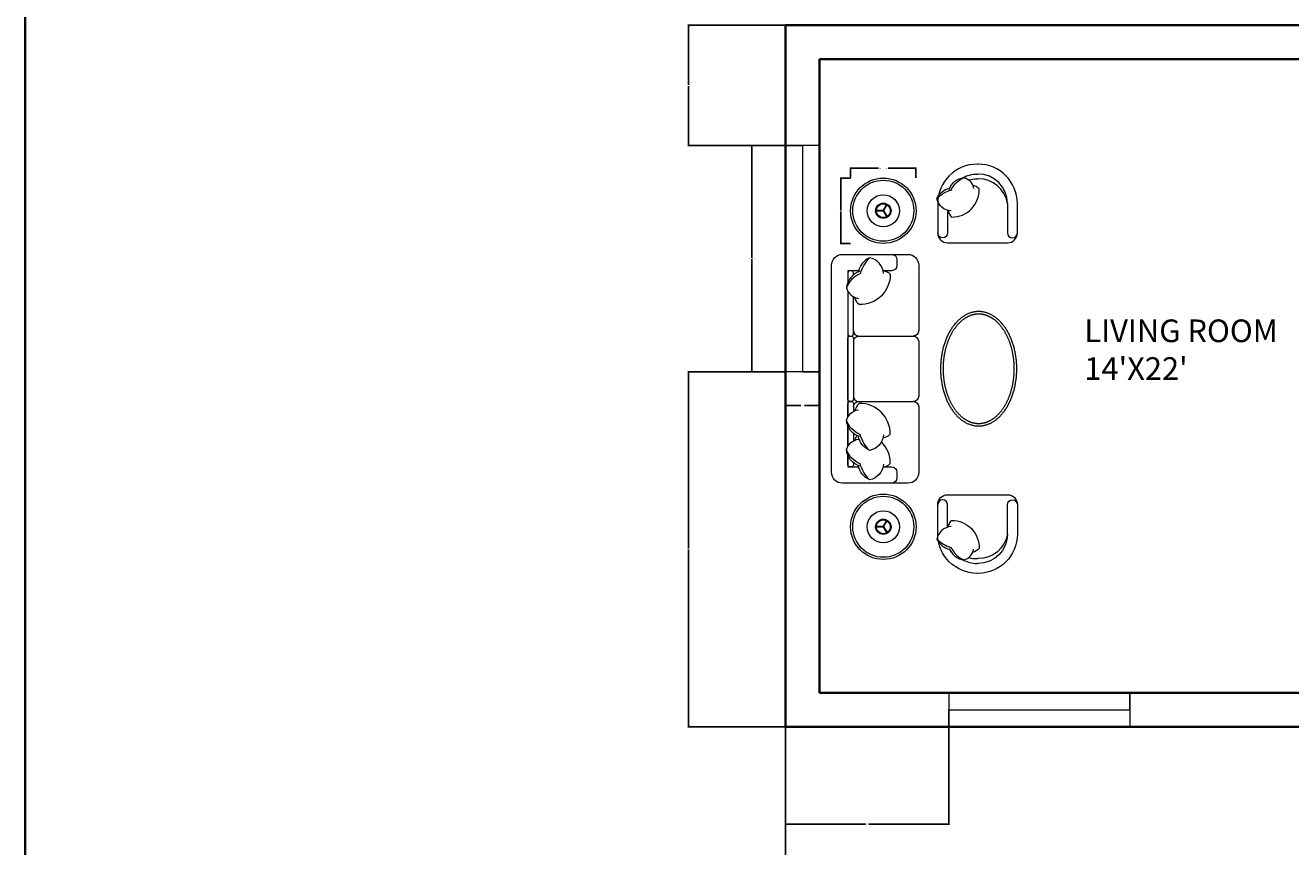
# Model space of a CAD drawing. Units: inches. Extents: x 2067 to 3463, y 1605 to 2723.
# Tile 2 of 10: x 2067 to 2403, y 1820 to 2038. Entities that reach past the tile are written whole.
import ezdxf

# ---------------------------------------------------------------- set-up
doc = ezdxf.new("R2010")
doc.units = ezdxf.units.IN
for name, color, linetype, lineweight in [('A-ANNO-DIMS', 2, 'Continuous', 18), ('A-ANNO-TTLB', 7, 'Continuous', 35), ('A-AREA-IDEN', 7, 'Continuous', 18), ('A-FURN', 8, 'Continuous', 13), ('A-GLAZ', 4, 'Continuous', 18), ('A-WALL', 7, 'Continuous', 35)]:
    doc.layers.add(name, color=color, linetype=linetype, lineweight=lineweight)
doc.styles.get("Standard").update_dxf_attribs({"font": 'arial.ttf'})
doc.dimstyles.get("Standard").update_dxf_attribs({"dimtxt": 0.18, "dimasz": 0.18, "dimexe": 0.18, "dimexo": 0.0625, "dimgap": 0.09, "dimtad": 0, "dimtih": 1, "dimtoh": 1, "dimdec": 4, "dimzin": 0, "dimdsep": 46, "dimtxsty": 'Standard', "dimcen": 0.09, "dimadec": 0, "dimazin": 0, "dimtfac": 1, "dimtdec": 4, "dimtofl": 0, "dimtmove": 0, "dimatfit": 3, "dimfxl": 1, "dimtolj": 1, "dimtzin": 0, "dimarcsym": 0})

# ---------------------------------------------------------------- blocks, each defined once
blk = doc.blocks.new('TABLE-SIDE-ROUND')
at = {"ltscale": 0.03}
for p, q in [((0, 0.09), (-2.04, 0.09)), ((-0.08, 0.05), (0.94, 1.81)), ((0.08, -0.05), (1.1, 1.72)), ((0.08, 0.05), (1.1, -1.72)), ((0, -0.09), (-2.04, -0.09)), ((-0.08, -0.05), (0.94, -1.81))]:
    blk.add_line(p, q, dxfattribs=at)
for radius in [8.67, 4.26, 2.04, 1.83]:
    blk.add_circle((0, 0), radius, dxfattribs=at)
blk.add_circle((0, 0), 8.09)
blk = doc.blocks.new('WIN-PLAN-60-OFFSET')
for p, q in [((0, 9), (0, 0)), ((60, 4.5), (60, 9)), ((60, 9), (60, 0)), ((0, 0), (0, 4.5)), ((0, 4.5), (60, 4.5))]:
    blk.add_line(p, q)
blk = doc.blocks.new('WIN-PLAN-48-OFFSET')
for p, q in [((0, 9), (0, 0)), ((48, 4.5), (48, 9)), ((48, 9), (48, 0)), ((0, 0), (0, 4.5)), ((0, 4.5), (48, 4.5))]:
    blk.add_line(p, q)
blk = doc.blocks.new('*D12')
at = {"layer": 'A-ANNO-DIMS', "color": 0, "lineweight": -2, "transparency": 16777216}
for p, q in [((2286.19, 1997.77), (2286.19, 2000.49)), ((2303.52, 1997.77), (2303.52, 2000.49)), ((2286.37, 2000.31), (2293.57, 2000.31)), ((2303.34, 2000.31), (2296.14, 2000.31))]:
    blk.add_line(p, q, dxfattribs=at)
at = {"layer": 'A-ANNO-DIMS', "color": 0, "transparency": 16777216}
for points in [[(2286.37, 2000.34), (2286.37, 2000.28), (2286.19, 2000.31)], [(2303.34, 2000.34), (2303.34, 2000.28), (2303.52, 2000.31)]]:
    blk.add_solid(points, dxfattribs=at)
at = {"layer": 'Defpoints', "color": 0, "transparency": 16777216}
for p in [(2286.19, 1997.71), (2303.52, 2000.31), (2303.52, 1997.71)]:
    blk.add_point(p, dxfattribs=at)
at = {"layer": 'A-ANNO-DIMS', "color": 0, "transparency": 16777216, "insert": (2294.86, 2000.31), "char_height": 0.18, "attachment_point": 5}
blk.add_mtext('\\A1;SIDE TABLE 17 TYP.', dxfattribs=at)
blk = doc.blocks.new('*D13')
at = {"layer": 'A-ANNO-DIMS', "color": 0, "lineweight": -2, "transparency": 16777216}
for p, q in [((2286.12, 1997.71), (2283.41, 1997.71)), ((2283.59, 1997.53), (2283.59, 1989.22)), ((2283.59, 1980.55), (2283.59, 1988.86)), ((2286.12, 1980.37), (2283.41, 1980.37))]:
    blk.add_line(p, q, dxfattribs=at)
at = {"layer": 'A-ANNO-DIMS', "color": 0, "transparency": 16777216}
for points in [[(2283.56, 1997.53), (2283.62, 1997.53), (2283.59, 1997.71)], [(2283.56, 1980.55), (2283.62, 1980.55), (2283.59, 1980.37)]]:
    blk.add_solid(points, dxfattribs=at)
at = {"layer": 'Defpoints', "color": 0, "transparency": 16777216}
for p in [(2283.59, 1997.71), (2286.19, 1997.71), (2286.19, 1980.37)]:
    blk.add_point(p, dxfattribs=at)
at = {"layer": 'A-ANNO-DIMS', "color": 0, "transparency": 16777216, "insert": (2283.59, 1989.04), "char_height": 0.18, "attachment_point": 5}
blk.add_mtext('\\A1;17 TYP.', dxfattribs=at)
blk = doc.blocks.new('*D22')
at = {"layer": 'A-ANNO-DIMS', "color": 0, "lineweight": -2, "transparency": 16777216}
for p, q in [((2268.89, 2006.36), (2259.77, 2006.36)), ((2259.95, 2006.18), (2259.95, 1976.54)), ((2259.95, 1946.54), (2259.95, 1976.18)), ((2268.89, 1946.36), (2259.77, 1946.36))]:
    blk.add_line(p, q, dxfattribs=at)
at = {"layer": 'A-ANNO-DIMS', "color": 0, "transparency": 16777216}
for points in [[(2259.92, 2006.18), (2259.98, 2006.18), (2259.95, 2006.36)], [(2259.92, 1946.54), (2259.98, 1946.54), (2259.95, 1946.36)]]:
    blk.add_solid(points, dxfattribs=at)
at = {"layer": 'Defpoints', "color": 0, "transparency": 16777216}
for p in [(2268.95, 2006.36), (2259.95, 1946.36), (2268.95, 1946.36)]:
    blk.add_point(p, dxfattribs=at)
at = {"layer": 'A-ANNO-DIMS', "color": 0, "transparency": 16777216, "insert": (2259.95, 1976.36), "char_height": 0.18, "attachment_point": 5}
blk.add_mtext('\\A1;WINDOW 60 TYP.', dxfattribs=at)
blk = doc.blocks.new('*D23')
at = {"layer": 'A-ANNO-DIMS', "color": 0, "lineweight": -2, "transparency": 16777216}
for p, q in [((2268.95, 1946.3), (2268.95, 1937.18)), ((2277.95, 1946.3), (2277.95, 1937.18)), ((2269.13, 1937.36), (2272.99, 1937.36)), ((2277.77, 1937.36), (2273.91, 1937.36))]:
    blk.add_line(p, q, dxfattribs=at)
at = {"layer": 'A-ANNO-DIMS', "color": 0, "transparency": 16777216}
for points in [[(2269.13, 1937.39), (2269.13, 1937.33), (2268.95, 1937.36)], [(2277.77, 1937.39), (2277.77, 1937.33), (2277.95, 1937.36)]]:
    blk.add_solid(points, dxfattribs=at)
at = {"layer": 'Defpoints', "color": 0, "transparency": 16777216}
for p in [(2268.95, 1946.36), (2277.95, 1946.36), (2277.95, 1937.36)]:
    blk.add_point(p, dxfattribs=at)
at = {"layer": 'A-ANNO-DIMS', "color": 0, "transparency": 16777216, "insert": (2273.45, 1937.36), "char_height": 0.18, "attachment_point": 5}
blk.add_mtext('\\A1;9 TYP.', dxfattribs=at)
blk = doc.blocks.new('*D32')
at = {"layer": 'A-ANNO-DIMS', "color": 0, "lineweight": -2, "transparency": 16777216}
for p, q in [((2268.89, 2038.22), (2242.97, 2038.22)), ((2243.15, 2038.04), (2243.15, 2022.47)), ((2243.15, 2006.54), (2243.15, 2022.11)), ((2268.89, 2006.36), (2242.97, 2006.36))]:
    blk.add_line(p, q, dxfattribs=at)
at = {"layer": 'A-ANNO-DIMS', "color": 0, "transparency": 16777216}
for points in [[(2243.12, 2038.04), (2243.18, 2038.04), (2243.15, 2038.22)], [(2243.12, 2006.54), (2243.18, 2006.54), (2243.15, 2006.36)]]:
    blk.add_solid(points, dxfattribs=at)
at = {"layer": 'Defpoints', "color": 0, "transparency": 16777216}
for p in [(2243.15, 2038.22), (2268.95, 2038.22), (2268.95, 2006.36)]:
    blk.add_point(p, dxfattribs=at)
at = {"layer": 'A-ANNO-DIMS', "color": 0, "transparency": 16777216, "insert": (2243.15, 2022.29), "char_height": 0.18, "attachment_point": 5}
blk.add_mtext('\\A1;31.86', dxfattribs=at)
blk = doc.blocks.new('*D33')
at = {"layer": 'A-ANNO-DIMS', "color": 0, "lineweight": -2, "transparency": 16777216}
for p, q in [((2268.89, 1946.36), (2242.97, 1946.36)), ((2243.15, 1946.18), (2243.15, 1899.47)), ((2243.15, 1852.4), (2243.15, 1899.11)), ((2268.89, 1852.22), (2242.97, 1852.22))]:
    blk.add_line(p, q, dxfattribs=at)
at = {"layer": 'A-ANNO-DIMS', "color": 0, "transparency": 16777216}
for points in [[(2243.12, 1946.18), (2243.18, 1946.18), (2243.15, 1946.36)], [(2243.12, 1852.4), (2243.18, 1852.4), (2243.15, 1852.22)]]:
    blk.add_solid(points, dxfattribs=at)
at = {"layer": 'Defpoints', "color": 0, "transparency": 16777216}
for p in [(2243.15, 1946.36), (2268.95, 1946.36), (2268.95, 1852.22)]:
    blk.add_point(p, dxfattribs=at)
at = {"layer": 'A-ANNO-DIMS', "color": 0, "transparency": 16777216, "insert": (2243.15, 1899.29), "char_height": 0.18, "attachment_point": 5}
blk.add_mtext('\\A1;94.14', dxfattribs=at)
blk = doc.blocks.new('*D36')
at = {"layer": 'A-ANNO-DIMS', "color": 0, "lineweight": -2, "transparency": 16777216}
for p, q in [((2268.95, 1852.15), (2268.95, 1764.75)), ((2433.25, 1806.19), (2433.25, 1764.75)), ((2269.13, 1764.93), (2350.71, 1764.93)), ((2433.07, 1764.93), (2351.49, 1764.93))]:
    blk.add_line(p, q, dxfattribs=at)
at = {"layer": 'A-ANNO-DIMS', "color": 0, "transparency": 16777216}
for points in [[(2269.13, 1764.96), (2269.13, 1764.9), (2268.95, 1764.93)], [(2433.07, 1764.96), (2433.07, 1764.9), (2433.25, 1764.93)]]:
    blk.add_solid(points, dxfattribs=at)
at = {"layer": 'Defpoints', "color": 0, "transparency": 16777216}
for p in [(2268.95, 1852.22), (2433.25, 1806.25), (2433.25, 1764.93)]:
    blk.add_point(p, dxfattribs=at)
at = {"layer": 'A-ANNO-DIMS', "color": 0, "transparency": 16777216, "insert": (2351.1, 1764.93), "char_height": 0.18, "attachment_point": 5}
blk.add_mtext('\\A1;164.3', dxfattribs=at)
blk = doc.blocks.new('*D42')
at = {"layer": 'A-ANNO-DIMS', "color": 0, "lineweight": -2, "transparency": 16777216}
for p, q in [((2268.95, 1852.15), (2268.95, 1826.24)), ((2312.26, 1852.15), (2312.26, 1826.24)), ((2269.13, 1826.42), (2290.22, 1826.42)), ((2312.08, 1826.42), (2290.98, 1826.42))]:
    blk.add_line(p, q, dxfattribs=at)
at = {"layer": 'A-ANNO-DIMS', "color": 0, "transparency": 16777216}
for points in [[(2269.13, 1826.45), (2269.13, 1826.39), (2268.95, 1826.42)], [(2312.08, 1826.45), (2312.08, 1826.39), (2312.26, 1826.42)]]:
    blk.add_solid(points, dxfattribs=at)
at = {"layer": 'Defpoints', "color": 0, "transparency": 16777216}
for p in [(2268.95, 1852.22), (2312.26, 1852.22), (2268.95, 1826.42)]:
    blk.add_point(p, dxfattribs=at)
at = {"layer": 'A-ANNO-DIMS', "color": 0, "transparency": 16777216, "insert": (2290.6, 1826.42), "char_height": 0.18, "attachment_point": 5}
blk.add_mtext('\\A1;43.31', dxfattribs=at)

msp = doc.modelspace()

# ---------------------------------------------------------------- linework, layer by layer
at = {"layer": 'A-ANNO-TTLB'}
msp.add_lwpolyline([(2067.2624, 2722.6321), (3463.3053, 2722.6321), (3463.3053, 1605.3918), (2067.2624, 1605.3918)], close=True, dxfattribs=at)
at = {"layer": 'A-FURN', "ltscale": 0.03}
for points in [[(2319.8521, 1980.5461), (2327.799, 1980.5461, 0.41421356), (2330.4045, 1983.1516), (2330.4045, 1990.9682, 0.41421356), (2319.9824, 2001.3903), (2319.8521, 2001.3903), (2319.7219, 2001.3903, 0.41421356), (2309.2997, 1990.9682), (2309.2997, 1983.1516, 0.41421356), (2311.9053, 1980.5461), (2319.8521, 1980.5461)], [(2319.8521, 1913.731), (2327.799, 1913.731, -0.41421356), (2330.4045, 1911.1254), (2330.4045, 1903.3089, -0.41421356), (2319.9824, 1892.8867), (2319.8521, 1892.8867), (2319.7219, 1892.8867, -0.41421356), (2309.2997, 1903.3089), (2309.2997, 1911.1254, -0.41421356), (2311.9053, 1913.731), (2319.8521, 1913.731)]]:
    msp.add_lwpolyline(points, format="xyb", dxfattribs=at)
at = {"layer": 'A-FURN'}
for points in [[(2309.0867, 1992.2833, -0.14772988), (2312.8943, 1994.5222, -0.21334276), (2316.2539, 1997.806, -0.17866181)], [(2312.3682, 1994.7007, -0.30666349), (2316.2539, 1997.806, -0.30632997), (2318.7923, 1994.97, 0.87284716)], [(2315.8418, 1997.7538, -0.13059149), (2319.7219, 1998.7848), (2319.8521, 1998.7848)], [(2317.5007, 1997.2013, -0.07238424), (2319.7219, 1997.482), (2319.8521, 1997.482)], [(2327.799, 1990.9682, 0.41421356), (2319.9824, 1998.7848), (2319.8521, 1998.7848)], [(2327.799, 1990.9682, 0.37271891), (2319.9824, 1997.482), (2319.8521, 1997.482)], [(2312.8196, 1988.9995, -0.35677236), (2309.0867, 1992.2833, -0.24954205), (2312.469, 1994.9894, 9.61688035)], [(2312.163, 1989.079, 0.16554063), (2312.9689, 1987.3576, 0.42598917), (2320.2855, 1994.8207, 0.12152332), (2318.5487, 1995.8494, -7.11546429)], [(2327.799, 1990.9683), (2327.799, 1983.1516, 0.41421356), (2329.1018, 1981.8489), (2329.1018, 1981.8489, 0.41421356), (2330.4045, 1983.1516)], [(2311.9053, 1989.1416), (2311.9053, 1983.1516, -0.41421356), (2310.6025, 1981.8489), (2310.6025, 1981.8489, -0.41421356), (2309.2997, 1983.1516)], [(2297.023, 1977.4811, -0.41421356), (2298.4678, 1976.0362), (2298.4678, 1974.5913, -0.41421356), (2297.023, 1973.1464), (2294.7843, 1973.1464)], [(2291.2298, 1976.5615, 0.14772988), (2288.7466, 1972.3385, 0.21334276), (2285.1046, 1968.6124, 0.17866181)], [(2294.8718, 1972.4213, 0.35677236), (2291.2298, 1976.5615, 0.24954205), (2288.2284, 1972.8101, -9.61688035)], [(2288.5487, 1972.922, 0.30666349), (2285.1046, 1968.6124, 0.30632997), (2288.2499, 1965.7971, -0.87284716)], [(2286.9088, 1972.0438), (2286.9088, 1972.5685, 0.41421356), (2286.3308, 1973.1464), (2286.0418, 1973.1464, 0.41421356), (2285.4639, 1972.5685)], [(2285.4639, 1972.5685), (2285.4639, 1970.1068, 0.41421356)], [(2294.7837, 1973.1496, -0.16554063), (2296.6928, 1972.2557, -0.42598917), (2288.4155, 1964.141, -0.12152332), (2287.2746, 1966.0673, 7.11546429)], [(2285.4639, 1967.703), (2285.4639, 1956.3858, 0.41421356), (2286.0418, 1955.8078), (2286.3308, 1955.8078, 0.41421356), (2286.9088, 1956.3858), (2286.9088, 1966.2481, 0.41421356)], [(2286.9088, 1957.2527, 0.41421356), (2288.3537, 1955.8078), (2302.8025, 1955.8078, 0.41421356)], [(2286.9088, 1954.363, -0.41421356), (2288.3537, 1955.8078)], [(2285.4639, 1934.3575), (2285.4639, 1937.8913, -0.41421356), (2286.0418, 1938.4692), (2286.3308, 1938.4692, -0.41421356), (2286.9088, 1937.8913), (2286.9088, 1935.8125, -0.41421356)], [(2286.9088, 1939.9141, 0.41421356), (2288.3537, 1938.4692)], [(2286.9088, 1937.0243, -0.41421356), (2288.3537, 1938.4692), (2302.8025, 1938.4692, -0.41421356)], [(2294.7837, 1928.911, 0.16554063), (2296.6928, 1929.8049, 0.42598917), (2288.4155, 1937.9196, 0.12152332), (2287.2746, 1935.9933, -7.11546429)], [(2288.5487, 1929.1386, -0.30666349), (2285.1046, 1933.4482, -0.30632997), (2288.2499, 1936.2635, 0.87284716)], [(2291.2298, 1925.4991, -0.14772988), (2288.7466, 1929.7221, -0.21334276), (2285.1046, 1933.4482, -0.17866181)], [(2285.4639, 1926.574), (2285.4639, 1931.9538, -0.41421356)], [(2286.9088, 1930.0168), (2286.9088, 1928.0289, -0.41421356)], [(2288.5487, 1921.3551, -0.30666349), (2285.1046, 1925.6647, -0.30632997), (2288.2499, 1928.48, 0.87284716)], [(2287.8395, 1929.4212, 0.07186538), (2287.2746, 1928.2098, -7.11546429)], [(2294.8718, 1929.6392, -0.35677236), (2291.2298, 1925.4991, -0.24954205), (2288.2284, 1929.2505, 9.61688035)], [(2294.7837, 1921.1275, 0.16554063), (2296.6928, 1922.0213, 0.20023115), (2294.3677, 1927.757, 0.12152332)], [(2291.2298, 1917.7155, -0.14772988), (2288.7466, 1921.9385, -0.21334276), (2285.1046, 1925.6647, -0.17866181)], [(2285.4639, 1924.1702), (2285.4639, 1921.1306), (2288.3034, 1921.1306, -0.41421356)], [(2285.4639, 1921.7086), (2285.4639, 1924.1702, -0.41421356)], [(2286.9088, 1922.2332), (2286.9088, 1921.7086, -0.41421356), (2286.3308, 1921.1306), (2286.0418, 1921.1306, -0.41421356), (2285.4639, 1921.7086)], [(2294.8718, 1921.8557, -0.35677236), (2291.2298, 1917.7155, -0.24954205), (2288.2284, 1921.4669, 9.61688035)], [(2294.7843, 1921.1306), (2297.023, 1921.1306, -0.41421356), (2298.4678, 1919.6857), (2298.4678, 1918.2408, -0.41421356), (2297.023, 1916.796)], [(2311.9053, 1905.1355), (2311.9053, 1911.1254, 0.41421356), (2310.6025, 1912.4282), (2310.6025, 1912.4282, 0.41421356), (2309.2997, 1911.1254)], [(2327.799, 1903.3087), (2327.799, 1911.1254, -0.41421356), (2329.1018, 1912.4282), (2329.1018, 1912.4282, -0.41421356), (2330.4045, 1911.1254)], [(2312.163, 1905.1981, -0.16554063), (2312.9689, 1906.9194, -0.42598917), (2320.2855, 1899.4563, -0.12152332), (2318.5487, 1898.4277, 7.11546429)], [(2312.8196, 1905.2775, 0.35677236), (2309.0867, 1901.9938, 0.24954205), (2312.469, 1899.2877, -9.61688035)], [(2327.799, 1903.3089, -0.37271891), (2319.9824, 1896.795), (2319.8521, 1896.795)], [(2327.799, 1903.3089, -0.41421356), (2319.9824, 1895.4923), (2319.8521, 1895.4923)], [(2309.0867, 1901.9938, 0.14772988), (2312.8943, 1899.7548, 0.21334276), (2316.2539, 1896.4711, 0.17866181)], [(2312.3682, 1899.5764, 0.30666349), (2316.2539, 1896.4711, 0.30632997), (2318.7923, 1899.307, -0.87284716)], [(2315.8418, 1896.5232, 0.13059149), (2319.7219, 1895.4923), (2319.8521, 1895.4923)], [(2317.5007, 1897.0757, 0.07238424), (2319.7219, 1896.795), (2319.8521, 1896.795)]]:
    msp.add_lwpolyline(points, format="xyb", dxfattribs=at)
at = {"layer": 'A-FURN', "ltscale": 0.03}
msp.add_lwpolyline([(2301.3576, 1977.4811, -0.41421356), (2304.2474, 1974.5913), (2304.2474, 1957.2527, -0.41421356), (2302.8025, 1955.8078, -0.41421356), (2304.2474, 1954.363), (2304.2474, 1939.9141, -0.41421356), (2302.8025, 1938.4692, -0.41421356), (2304.2474, 1937.0243), (2304.2474, 1919.6857, -0.41421356), (2301.3576, 1916.796), (2284.019, 1916.796, -0.41421356), (2281.1292, 1919.6857), (2281.1292, 1974.5913, -0.41421356), (2284.019, 1977.4811)], format="xyb", close=True, dxfattribs=at)
at = {"layer": 'A-FURN'}
for points in [[(2288.3034, 1973.1464), (2285.4639, 1973.1464), (2285.4639, 1970.1068)], [(2285.4639, 1967.703), (2285.4639, 1934.3575)], [(2285.4639, 1931.9538), (2285.4639, 1926.574)]]:
    msp.add_lwpolyline(points, dxfattribs=at)
msp.add_lwpolyline([(2285.4639, 1939.0472), (2285.4639, 1955.2299, -0.41421356), (2286.0418, 1955.8078), (2286.3308, 1955.8078, -0.41421356), (2286.9088, 1955.2299), (2286.9088, 1939.0472, -0.41421356), (2286.3308, 1938.4692), (2286.0418, 1938.4692, -0.41421356)], format="xyb", close=True, dxfattribs=at)
at = {"layer": 'A-FURN', "ltscale": 0.03}
msp.add_polyline3d([(2320.1411, 1962.3098, 0), (2319.9497, 1962.3071, 0), (2319.7584, 1962.2989, 0), (2319.5672, 1962.2854, 0), (2319.3762, 1962.2664, 0), (2319.1855, 1962.2419, 0), (2318.9951, 1962.2121, 0), (2318.8051, 1962.1769, 0), (2318.6156, 1962.1363, 0), (2318.4267, 1962.0903, 0), (2318.2384, 1962.0389, 0), (2318.0507, 1961.9823, 0), (2317.8638, 1961.9203, 0), (2317.6778, 1961.853, 0), (2317.4926, 1961.7804, 0), (2317.3083, 1961.7026, 0), (2317.1251, 1961.6196, 0), (2316.9429, 1961.5314, 0), (2316.7619, 1961.438, 0), (2316.5821, 1961.3395, 0), (2316.4036, 1961.236, 0), (2316.2264, 1961.1273, 0), (2316.0506, 1961.0137, 0), (2315.8763, 1960.8951, 0), (2315.7035, 1960.7716, 0), (2315.5323, 1960.6432, 0), (2315.3628, 1960.5099, 0), (2315.1949, 1960.3719, 0), (2315.0289, 1960.2291, 0), (2314.8646, 1960.0817, 0), (2314.7023, 1959.9296, 0), (2314.5419, 1959.7729, 0), (2314.3835, 1959.6117, 0), (2314.2272, 1959.446, 0), (2314.0729, 1959.2759, 0), (2313.9209, 1959.1015, 0), (2313.7711, 1958.9228, 0), (2313.6236, 1958.7399, 0), (2313.4784, 1958.5528, 0), (2313.3356, 1958.3616, 0), (2313.1952, 1958.1664, 0), (2313.0573, 1957.9673, 0), (2312.9219, 1957.7643, 0), (2312.7892, 1957.5574, 0), (2312.6591, 1957.3469, 0), (2312.5316, 1957.1327, 0), (2312.4069, 1956.9149, 0), (2312.2849, 1956.6936, 0), (2312.1658, 1956.4688, 0), (2312.0495, 1956.2408, 0), (2311.9361, 1956.0095, 0), (2311.8257, 1955.775, 0), (2311.7182, 1955.5374, 0), (2311.6137, 1955.2968, 0), (2311.5124, 1955.0533, 0), (2311.414, 1954.8069, 0), (2311.3189, 1954.5578, 0), (2311.2268, 1954.306, 0), (2311.138, 1954.0517, 0), (2311.0524, 1953.7949, 0), (2310.9701, 1953.5357, 0), (2310.891, 1953.2743, 0), (2310.8152, 1953.0106, 0), (2310.7428, 1952.7448, 0), (2310.6738, 1952.477, 0), (2310.6081, 1952.2073, 0), (2310.5459, 1951.9358, 0), (2310.4871, 1951.6626, 0), (2310.4317, 1951.3877, 0), (2310.3799, 1951.1113, 0), (2310.3315, 1950.8336, 0), (2310.2866, 1950.5544, 0), (2310.2453, 1950.2741, 0), (2310.2075, 1949.9926, 0), (2310.1733, 1949.7101, 0), (2310.1426, 1949.4267, 0), (2310.1155, 1949.1425, 0), (2310.0921, 1948.8576, 0), (2310.0722, 1948.572, 0), (2310.0559, 1948.2859, 0), (2310.0432, 1947.9994, 0), (2310.0342, 1947.7126, 0), (2310.0287, 1947.4256, 0), (2310.0269, 1947.1385, 0), (2310.0287, 1946.8514, 0), (2310.0342, 1946.5644, 0), (2310.0432, 1946.2776, 0), (2310.0559, 1945.9911, 0), (2310.0722, 1945.7051, 0), (2310.0921, 1945.4195, 0), (2310.1155, 1945.1346, 0), (2310.1426, 1944.8503, 0), (2310.1733, 1944.5669, 0), (2310.2075, 1944.2844, 0), (2310.2453, 1944.003, 0), (2310.2866, 1943.7226, 0), (2310.3315, 1943.4435, 0), (2310.3799, 1943.1657, 0), (2310.4317, 1942.8893, 0), (2310.4871, 1942.6145, 0), (2310.5459, 1942.3413, 0), (2310.6081, 1942.0697, 0), (2310.6738, 1941.8, 0), (2310.7428, 1941.5323, 0), (2310.8152, 1941.2665, 0), (2310.891, 1941.0028, 0), (2310.9701, 1940.7413, 0), (2311.0524, 1940.4821, 0), (2311.138, 1940.2253, 0), (2311.2268, 1939.971, 0), (2311.3189, 1939.7193, 0), (2311.414, 1939.4702, 0), (2311.5124, 1939.2238, 0), (2311.6137, 1938.9803, 0), (2311.7182, 1938.7397, 0), (2311.8257, 1938.5021, 0), (2311.9361, 1938.2676, 0), (2312.0495, 1938.0363, 0), (2312.1658, 1937.8082, 0), (2312.2849, 1937.5835, 0), (2312.4069, 1937.3622, 0), (2312.5316, 1937.1444, 0), (2312.6591, 1936.9302, 0), (2312.7892, 1936.7196, 0), (2312.9219, 1936.5128, 0), (2313.0573, 1936.3098, 0), (2313.1952, 1936.1106, 0), (2313.3356, 1935.9154, 0), (2313.4784, 1935.7243, 0), (2313.6236, 1935.5372, 0), (2313.7711, 1935.3543, 0), (2313.9209, 1935.1755, 0), (2314.0729, 1935.0011, 0), (2314.2272, 1934.831, 0), (2314.3835, 1934.6654, 0), (2314.5419, 1934.5042, 0), (2314.7023, 1934.3475, 0), (2314.8646, 1934.1954, 0), (2315.0289, 1934.0479, 0), (2315.1949, 1933.9052, 0), (2315.3628, 1933.7671, 0), (2315.5323, 1933.6339, 0), (2315.7035, 1933.5055, 0), (2315.8763, 1933.3819, 0), (2316.0506, 1933.2633, 0), (2316.2264, 1933.1497, 0), (2316.4036, 1933.0411, 0), (2316.5821, 1932.9375, 0), (2316.7619, 1932.839, 0), (2316.9429, 1932.7457, 0), (2317.1251, 1932.6575, 0), (2317.3083, 1932.5745, 0), (2317.4926, 1932.4967, 0), (2317.6778, 1932.4241, 0), (2317.8638, 1932.3568, 0), (2318.0507, 1932.2948, 0), (2318.2384, 1932.2381, 0), (2318.4267, 1932.1868, 0), (2318.6156, 1932.1408, 0), (2318.8051, 1932.1002, 0), (2318.9951, 1932.0649, 0), (2319.1855, 1932.0351, 0), (2319.3762, 1932.0107, 0), (2319.5672, 1931.9917, 0), (2319.7584, 1931.9781, 0), (2319.9497, 1931.97, 0), (2320.1411, 1931.9672, 0), (2320.3325, 1931.97, 0), (2320.5238, 1931.9781, 0), (2320.715, 1931.9917, 0), (2320.906, 1932.0107, 0), (2321.0968, 1932.0351, 0), (2321.2871, 1932.0649, 0), (2321.4771, 1932.1002, 0), (2321.6666, 1932.1408, 0), (2321.8555, 1932.1868, 0), (2322.0438, 1932.2381, 0), (2322.2315, 1932.2948, 0), (2322.4184, 1932.3568, 0), (2322.6045, 1932.4241, 0), (2322.7897, 1932.4967, 0), (2322.9739, 1932.5745, 0), (2323.1571, 1932.6575, 0), (2323.3393, 1932.7457, 0), (2323.5203, 1932.839, 0), (2323.7001, 1932.9375, 0), (2323.8786, 1933.0411, 0), (2324.0558, 1933.1497, 0), (2324.2316, 1933.2633, 0), (2324.4059, 1933.3819, 0), (2324.5787, 1933.5055, 0), (2324.7499, 1933.6339, 0), (2324.9195, 1933.7671, 0), (2325.0873, 1933.9052, 0), (2325.2534, 1934.0479, 0), (2325.4176, 1934.1954, 0), (2325.5799, 1934.3475, 0), (2325.7403, 1934.5042, 0), (2325.8987, 1934.6654, 0), (2326.0551, 1934.831, 0), (2326.2093, 1935.0011, 0), (2326.3613, 1935.1755, 0), (2326.5111, 1935.3543, 0), (2326.6587, 1935.5372, 0), (2326.8039, 1935.7243, 0), (2326.9467, 1935.9154, 0), (2327.087, 1936.1106, 0), (2327.2249, 1936.3098, 0), (2327.3603, 1936.5128, 0), (2327.493, 1936.7196, 0), (2327.6232, 1936.9302, 0), (2327.7506, 1937.1444, 0), (2327.8753, 1937.3622, 0), (2327.9973, 1937.5835, 0), (2328.1164, 1937.8082, 0), (2328.2327, 1938.0363, 0), (2328.3461, 1938.2676, 0), (2328.4566, 1938.5021, 0), (2328.564, 1938.7397, 0), (2328.6685, 1938.9803, 0), (2328.7699, 1939.2238, 0), (2328.8682, 1939.4702, 0), (2328.9634, 1939.7193, 0), (2329.0554, 1939.971, 0), (2329.1442, 1940.2253, 0), (2329.2298, 1940.4821, 0), (2329.3122, 1940.7413, 0), (2329.3912, 1941.0028, 0), (2329.467, 1941.2665, 0), (2329.5394, 1941.5323, 0), (2329.6084, 1941.8, 0), (2329.6741, 1942.0697, 0), (2329.7363, 1942.3413, 0), (2329.7951, 1942.6145, 0), (2329.8505, 1942.8893, 0), (2329.9024, 1943.1657, 0), (2329.9507, 1943.4435, 0), (2329.9956, 1943.7226, 0), (2330.0369, 1944.003, 0), (2330.0747, 1944.2844, 0), (2330.1089, 1944.5669, 0), (2330.1396, 1944.8503, 0), (2330.1667, 1945.1346, 0), (2330.1902, 1945.4195, 0), (2330.2101, 1945.7051, 0), (2330.2263, 1945.9911, 0), (2330.239, 1946.2776, 0), (2330.2481, 1946.5644, 0), (2330.2535, 1946.8514, 0), (2330.2553, 1947.1385, 0), (2330.2535, 1947.4256, 0), (2330.2481, 1947.7126, 0), (2330.239, 1947.9994, 0), (2330.2263, 1948.2859, 0), (2330.2101, 1948.572, 0), (2330.1902, 1948.8576, 0), (2330.1667, 1949.1425, 0), (2330.1396, 1949.4267, 0), (2330.1089, 1949.7101, 0), (2330.0747, 1949.9926, 0), (2330.0369, 1950.2741, 0), (2329.9956, 1950.5544, 0), (2329.9507, 1950.8336, 0), (2329.9024, 1951.1113, 0), (2329.8505, 1951.3877, 0), (2329.7951, 1951.6626, 0), (2329.7363, 1951.9358, 0), (2329.6741, 1952.2073, 0), (2329.6084, 1952.477, 0), (2329.5394, 1952.7448, 0), (2329.467, 1953.0106, 0), (2329.3912, 1953.2743, 0), (2329.3122, 1953.5357, 0), (2329.2298, 1953.7949, 0), (2329.1442, 1954.0517, 0), (2329.0554, 1954.306, 0), (2328.9634, 1954.5578, 0), (2328.8682, 1954.8069, 0), (2328.7699, 1955.0533, 0), (2328.6685, 1955.2968, 0), (2328.564, 1955.5374, 0), (2328.4566, 1955.775, 0), (2328.3461, 1956.0095, 0), (2328.2327, 1956.2408, 0), (2328.1164, 1956.4688, 0), (2327.9973, 1956.6936, 0), (2327.8753, 1956.9149, 0), (2327.7506, 1957.1327, 0), (2327.6232, 1957.3469, 0), (2327.493, 1957.5574, 0), (2327.3603, 1957.7643, 0), (2327.2249, 1957.9673, 0), (2327.087, 1958.1664, 0), (2326.9467, 1958.3616, 0), (2326.8039, 1958.5528, 0), (2326.6587, 1958.7399, 0), (2326.5111, 1958.9228, 0), (2326.3613, 1959.1015, 0), (2326.2093, 1959.2759, 0), (2326.0551, 1959.446, 0), (2325.8987, 1959.6117, 0), (2325.7403, 1959.7729, 0), (2325.5799, 1959.9296, 0), (2325.4176, 1960.0817, 0), (2325.2534, 1960.2291, 0), (2325.0873, 1960.3719, 0), (2324.9195, 1960.5099, 0), (2324.7499, 1960.6432, 0), (2324.5787, 1960.7716, 0), (2324.4059, 1960.8951, 0), (2324.2316, 1961.0137, 0), (2324.0558, 1961.1273, 0), (2323.8786, 1961.236, 0), (2323.7001, 1961.3395, 0), (2323.5203, 1961.438, 0), (2323.3393, 1961.5314, 0), (2323.1571, 1961.6196, 0), (2322.9739, 1961.7026, 0), (2322.7897, 1961.7804, 0), (2322.6045, 1961.853, 0), (2322.4184, 1961.9203, 0), (2322.2315, 1961.9823, 0), (2322.0438, 1962.0389, 0), (2321.8555, 1962.0903, 0), (2321.6666, 1962.1363, 0), (2321.4771, 1962.1769, 0), (2321.2871, 1962.2121, 0), (2321.0968, 1962.2419, 0), (2320.906, 1962.2664, 0), (2320.715, 1962.2854, 0), (2320.5238, 1962.2989, 0), (2320.3325, 1962.3071, 0), (2320.1411, 1962.3098, 0)], dxfattribs=at)
at = {"layer": 'A-FURN'}
msp.add_polyline3d([(2320.1411, 1961.6355, 0), (2320.0377, 1961.6347, 0), (2319.9338, 1961.632, 0), (2319.8294, 1961.6275, 0), (2319.7246, 1961.6212, 0), (2319.6193, 1961.6131, 0), (2319.5136, 1961.603, 0), (2319.4075, 1961.5911, 0), (2319.3011, 1961.5772, 0), (2319.1942, 1961.5614, 0), (2319.087, 1961.5437, 0), (2318.9794, 1961.5239, 0), (2318.8715, 1961.5021, 0), (2318.7633, 1961.4783, 0), (2318.6548, 1961.4524, 0), (2318.546, 1961.4245, 0), (2318.4369, 1961.3944, 0), (2318.3276, 1961.3622, 0), (2318.218, 1961.3278, 0), (2318.1081, 1961.2913, 0), (2317.9981, 1961.2525, 0), (2317.8879, 1961.2115, 0), (2317.7775, 1961.1683, 0), (2317.6669, 1961.1227, 0), (2317.5563, 1961.0749, 0), (2317.4455, 1961.0247, 0), (2317.3348, 1960.9723, 0), (2317.224, 1960.9176, 0), (2317.1133, 1960.8606, 0), (2317.0026, 1960.8012, 0), (2316.892, 1960.7396, 0), (2316.7816, 1960.6756, 0), (2316.6713, 1960.6093, 0), (2316.5612, 1960.5407, 0), (2316.4513, 1960.4697, 0), (2316.3417, 1960.3965, 0), (2316.2324, 1960.3209, 0), (2316.1234, 1960.243, 0), (2316.0147, 1960.1627, 0), (2315.9065, 1960.0801, 0), (2315.7986, 1959.9951, 0), (2315.6913, 1959.9078, 0), (2315.5844, 1959.8181, 0), (2315.478, 1959.7259, 0), (2315.3722, 1959.6312, 0), (2315.2669, 1959.534, 0), (2315.1622, 1959.4344, 0), (2315.0582, 1959.3323, 0), (2314.9548, 1959.2279, 0), (2314.8521, 1959.1211, 0), (2314.7501, 1959.0121, 0), (2314.6488, 1958.9007, 0), (2314.5483, 1958.7871, 0), (2314.4486, 1958.6713, 0), (2314.3496, 1958.5534, 0), (2314.2516, 1958.4333, 0), (2314.1544, 1958.3111, 0), (2314.0581, 1958.1869, 0), (2313.9627, 1958.0606, 0), (2313.8683, 1957.9324, 0), (2313.7749, 1957.8022, 0), (2313.6825, 1957.6701, 0), (2313.5911, 1957.5361, 0), (2313.5008, 1957.4002, 0), (2313.4116, 1957.2626, 0), (2313.3235, 1957.1231, 0), (2313.2365, 1956.9819, 0), (2313.1507, 1956.8391, 0), (2313.0662, 1956.6945, 0), (2312.9828, 1956.5483, 0), (2312.9007, 1956.4005, 0), (2312.8199, 1956.2511, 0), (2312.7405, 1956.1002, 0), (2312.6623, 1955.9479, 0), (2312.5856, 1955.794, 0), (2312.5102, 1955.6387, 0), (2312.4363, 1955.4821, 0), (2312.3638, 1955.3241, 0), (2312.2928, 1955.1647, 0), (2312.2233, 1955.0041, 0), (2312.1553, 1954.8422, 0), (2312.0889, 1954.6792, 0), (2312.0241, 1954.5149, 0), (2311.9609, 1954.3495, 0), (2311.8993, 1954.1832, 0), (2311.8394, 1954.0165, 0), (2311.7811, 1953.8492, 0), (2311.7244, 1953.6816, 0), (2311.6694, 1953.5135, 0), (2311.6159, 1953.345, 0), (2311.564, 1953.176, 0), (2311.5138, 1953.0067, 0), (2311.4651, 1952.837, 0), (2311.418, 1952.6669, 0), (2311.3724, 1952.4965, 0), (2311.3285, 1952.3257, 0), (2311.286, 1952.1545, 0), (2311.2452, 1951.983, 0), (2311.2058, 1951.8112, 0), (2311.168, 1951.6391, 0), (2311.1318, 1951.4667, 0), (2311.097, 1951.2941, 0), (2311.0638, 1951.1211, 0), (2311.0321, 1950.9479, 0), (2311.0018, 1950.7744, 0), (2310.9731, 1950.6008, 0), (2310.9459, 1950.4268, 0), (2310.9201, 1950.2527, 0), (2310.8958, 1950.0783, 0), (2310.873, 1949.9038, 0), (2310.8516, 1949.7291, 0), (2310.8317, 1949.5542, 0), (2310.8132, 1949.3792, 0), (2310.7962, 1949.204, 0), (2310.7805, 1949.0287, 0), (2310.7664, 1948.8532, 0), (2310.7536, 1948.6777, 0), (2310.7422, 1948.502, 0), (2310.7323, 1948.3263, 0), (2310.7237, 1948.1504, 0), (2310.7165, 1947.9745, 0), (2310.7107, 1947.7986, 0), (2310.7063, 1947.6226, 0), (2310.7033, 1947.4466, 0), (2310.7016, 1947.2706, 0), (2310.7012, 1947.0945, 0), (2310.7023, 1946.9185, 0), (2310.7046, 1946.7424, 0), (2310.7084, 1946.5664, 0), (2310.7135, 1946.3905, 0), (2310.72, 1946.2146, 0), (2310.7278, 1946.0387, 0), (2310.7371, 1945.8629, 0), (2310.7477, 1945.6872, 0), (2310.7598, 1945.5116, 0), (2310.7733, 1945.3361, 0), (2310.7882, 1945.1607, 0), (2310.8045, 1944.9855, 0), (2310.8223, 1944.8103, 0), (2310.8415, 1944.6354, 0), (2310.8621, 1944.4606, 0), (2310.8842, 1944.286, 0), (2310.9078, 1944.1115, 0), (2310.9328, 1943.9373, 0), (2310.9593, 1943.7632, 0), (2310.9873, 1943.5894, 0), (2311.0168, 1943.4158, 0), (2311.0477, 1943.2425, 0), (2311.0802, 1943.0694, 0), (2311.1142, 1942.8966, 0), (2311.1497, 1942.7241, 0), (2311.1867, 1942.5518, 0), (2311.2253, 1942.3799, 0), (2311.2654, 1942.2082, 0), (2311.3071, 1942.0369, 0), (2311.3503, 1941.866, 0), (2311.395, 1941.6953, 0), (2311.4413, 1941.5251, 0), (2311.4892, 1941.3552, 0), (2311.5387, 1941.1856, 0), (2311.5898, 1941.0165, 0), (2311.6424, 1940.8478, 0), (2311.6967, 1940.6795, 0), (2311.7526, 1940.5116, 0), (2311.8101, 1940.3441, 0), (2311.8692, 1940.1772, 0), (2311.9299, 1940.0106, 0), (2311.9923, 1939.8447, 0), (2312.0563, 1939.6799, 0), (2312.1219, 1939.5162, 0), (2312.1891, 1939.3537, 0), (2312.2578, 1939.1925, 0), (2312.3281, 1939.0325, 0), (2312.3998, 1938.8738, 0), (2312.473, 1938.7165, 0), (2312.5477, 1938.5605, 0), (2312.6238, 1938.4059, 0), (2312.7012, 1938.2528, 0), (2312.78, 1938.1012, 0), (2312.8602, 1937.951, 0), (2312.9416, 1937.8025, 0), (2313.0243, 1937.6555, 0), (2313.1083, 1937.5101, 0), (2313.1935, 1937.3664, 0), (2313.2798, 1937.2243, 0), (2313.3674, 1937.084, 0), (2313.456, 1936.9454, 0), (2313.5458, 1936.8087, 0), (2313.6366, 1936.6737, 0), (2313.7285, 1936.5407, 0), (2313.8215, 1936.4095, 0), (2313.9154, 1936.2803, 0), (2314.0103, 1936.153, 0), (2314.1061, 1936.0278, 0), (2314.2029, 1935.9046, 0), (2314.3005, 1935.7834, 0), (2314.399, 1935.6644, 0), (2314.4983, 1935.5475, 0), (2314.5984, 1935.4329, 0), (2314.6993, 1935.3204, 0), (2314.801, 1935.2102, 0), (2314.9033, 1935.1022, 0), (2315.0064, 1934.9966, 0), (2315.1101, 1934.8934, 0), (2315.2145, 1934.7925, 0), (2315.3195, 1934.6941, 0), (2315.425, 1934.5982, 0), (2315.5311, 1934.5047, 0), (2315.6377, 1934.4138, 0), (2315.7449, 1934.3253, 0), (2315.8525, 1934.2392, 0), (2315.9605, 1934.1554, 0), (2316.069, 1934.0739, 0), (2316.1778, 1933.9948, 0), (2316.287, 1933.9181, 0), (2316.3965, 1933.8436, 0), (2316.5062, 1933.7715, 0), (2316.6162, 1933.7018, 0), (2316.7264, 1933.6343, 0), (2316.8368, 1933.5692, 0), (2316.9473, 1933.5064, 0), (2317.0579, 1933.4459, 0), (2317.1686, 1933.3877, 0), (2317.2794, 1933.3318, 0), (2317.3902, 1933.2782, 0), (2317.5009, 1933.227, 0), (2317.6116, 1933.178, 0), (2317.7222, 1933.1313, 0), (2317.8327, 1933.0869, 0), (2317.943, 1933.0448, 0), (2318.0532, 1933.0049, 0), (2318.1631, 1932.9673, 0), (2318.2728, 1932.9318, 0), (2318.3823, 1932.8985, 0), (2318.4915, 1932.8674, 0), (2318.6004, 1932.8383, 0), (2318.7091, 1932.8114, 0), (2318.8175, 1932.7866, 0), (2318.9255, 1932.7638, 0), (2319.0332, 1932.743, 0), (2319.1406, 1932.7242, 0), (2319.2477, 1932.7075, 0), (2319.3543, 1932.6926, 0), (2319.4606, 1932.6798, 0), (2319.5665, 1932.6688, 0), (2319.672, 1932.6597, 0), (2319.777, 1932.6525, 0), (2319.8816, 1932.6471, 0), (2319.9858, 1932.6435, 0), (2320.0895, 1932.6417, 0), (2320.1928, 1932.6417, 0), (2320.2964, 1932.6435, 0), (2320.4006, 1932.6471, 0), (2320.5052, 1932.6525, 0), (2320.6102, 1932.6597, 0), (2320.7157, 1932.6688, 0), (2320.8216, 1932.6798, 0), (2320.9279, 1932.6926, 0), (2321.0346, 1932.7075, 0), (2321.1416, 1932.7242, 0), (2321.249, 1932.743, 0), (2321.3567, 1932.7638, 0), (2321.4648, 1932.7866, 0), (2321.5731, 1932.8114, 0), (2321.6818, 1932.8383, 0), (2321.7908, 1932.8674, 0), (2321.9, 1932.8985, 0), (2322.0094, 1932.9318, 0), (2322.1191, 1932.9673, 0), (2322.2291, 1933.0049, 0), (2322.3392, 1933.0448, 0), (2322.4495, 1933.0869, 0), (2322.56, 1933.1313, 0), (2322.6706, 1933.178, 0), (2322.7813, 1933.227, 0), (2322.8921, 1933.2782, 0), (2323.0028, 1933.3318, 0), (2323.1136, 1933.3877, 0), (2323.2243, 1933.4459, 0), (2323.3349, 1933.5064, 0), (2323.4454, 1933.5692, 0), (2323.5558, 1933.6343, 0), (2323.666, 1933.7018, 0), (2323.776, 1933.7715, 0), (2323.8858, 1933.8436, 0), (2323.9952, 1933.9181, 0), (2324.1044, 1933.9948, 0), (2324.2132, 1934.0739, 0), (2324.3217, 1934.1554, 0), (2324.4297, 1934.2392, 0), (2324.5373, 1934.3253, 0), (2324.6445, 1934.4138, 0), (2324.7511, 1934.5047, 0), (2324.8572, 1934.5982, 0), (2324.9628, 1934.6941, 0), (2325.0677, 1934.7925, 0), (2325.1721, 1934.8934, 0), (2325.2758, 1934.9966, 0), (2325.3789, 1935.1022, 0), (2325.4812, 1935.2102, 0), (2325.5829, 1935.3204, 0), (2325.6838, 1935.4329, 0), (2325.7839, 1935.5475, 0), (2325.8832, 1935.6644, 0), (2325.9817, 1935.7834, 0), (2326.0794, 1935.9046, 0), (2326.1761, 1936.0278, 0), (2326.2719, 1936.153, 0), (2326.3668, 1936.2803, 0), (2326.4607, 1936.4095, 0), (2326.5537, 1936.5407, 0), (2326.6456, 1936.6737, 0), (2326.7364, 1936.8087, 0), (2326.8262, 1936.9454, 0), (2326.9149, 1937.084, 0), (2327.0024, 1937.2243, 0), (2327.0888, 1937.3664, 0), (2327.1739, 1937.5101, 0), (2327.2579, 1937.6555, 0), (2327.3406, 1937.8025, 0), (2327.422, 1937.951, 0), (2327.5022, 1938.1012, 0), (2327.581, 1938.2528, 0), (2327.6584, 1938.4059, 0), (2327.7345, 1938.5605, 0), (2327.8092, 1938.7165, 0), (2327.8824, 1938.8738, 0), (2327.9542, 1939.0325, 0), (2328.0244, 1939.1925, 0), (2328.0932, 1939.3537, 0), (2328.1603, 1939.5162, 0), (2328.2259, 1939.6799, 0), (2328.29, 1939.8447, 0), (2328.3523, 1940.0106, 0), (2328.4131, 1940.1772, 0), (2328.4722, 1940.3441, 0), (2328.5297, 1940.5116, 0), (2328.5855, 1940.6795, 0), (2328.6398, 1940.8478, 0), (2328.6924, 1941.0165, 0), (2328.7435, 1941.1856, 0), (2328.793, 1941.3552, 0), (2328.8409, 1941.5251, 0), (2328.8872, 1941.6953, 0), (2328.932, 1941.866, 0), (2328.9752, 1942.0369, 0), (2329.0168, 1942.2082, 0), (2329.0569, 1942.3799, 0), (2329.0955, 1942.5518, 0), (2329.1325, 1942.7241, 0), (2329.168, 1942.8966, 0), (2329.202, 1943.0694, 0), (2329.2345, 1943.2425, 0), (2329.2655, 1943.4158, 0), (2329.2949, 1943.5894, 0), (2329.3229, 1943.7632, 0), (2329.3494, 1943.9373, 0), (2329.3745, 1944.1115, 0), (2329.398, 1944.286, 0), (2329.4201, 1944.4606, 0), (2329.4408, 1944.6354, 0), (2329.46, 1944.8103, 0), (2329.4777, 1944.9855, 0), (2329.4941, 1945.1607, 0), (2329.5089, 1945.3361, 0), (2329.5224, 1945.5116, 0), (2329.5345, 1945.6872, 0), (2329.5451, 1945.8629, 0), (2329.5544, 1946.0387, 0), (2329.5623, 1946.2146, 0), (2329.5688, 1946.3905, 0), (2329.5739, 1946.5664, 0), (2329.5776, 1946.7424, 0), (2329.58, 1946.9185, 0), (2329.581, 1947.0945, 0), (2329.5806, 1947.2706, 0), (2329.579, 1947.4466, 0), (2329.5759, 1947.6226, 0), (2329.5715, 1947.7986, 0), (2329.5657, 1947.9745, 0), (2329.5585, 1948.1504, 0), (2329.55, 1948.3263, 0), (2329.54, 1948.502, 0), (2329.5286, 1948.6777, 0), (2329.5159, 1948.8532, 0), (2329.5017, 1949.0287, 0), (2329.4861, 1949.204, 0), (2329.469, 1949.3792, 0), (2329.4506, 1949.5542, 0), (2329.4306, 1949.7291, 0), (2329.4093, 1949.9038, 0), (2329.3864, 1950.0783, 0), (2329.3621, 1950.2527, 0), (2329.3364, 1950.4268, 0), (2329.3091, 1950.6008, 0), (2329.2804, 1950.7744, 0), (2329.2502, 1950.9479, 0), (2329.2184, 1951.1211, 0), (2329.1852, 1951.2941, 0), (2329.1505, 1951.4667, 0), (2329.1142, 1951.6391, 0), (2329.0764, 1951.8112, 0), (2329.0371, 1951.983, 0), (2328.9962, 1952.1545, 0), (2328.9538, 1952.3257, 0), (2328.9098, 1952.4965, 0), (2328.8642, 1952.6669, 0), (2328.8171, 1952.837, 0), (2328.7684, 1953.0067, 0), (2328.7182, 1953.176, 0), (2328.6663, 1953.345, 0), (2328.6129, 1953.5135, 0), (2328.5578, 1953.6816, 0), (2328.5011, 1953.8492, 0), (2328.4428, 1954.0165, 0), (2328.3829, 1954.1832, 0), (2328.3213, 1954.3495, 0), (2328.2582, 1954.5149, 0), (2328.1933, 1954.6792, 0), (2328.1269, 1954.8422, 0), (2328.059, 1955.0041, 0), (2327.9895, 1955.1647, 0), (2327.9185, 1955.3241, 0), (2327.846, 1955.4821, 0), (2327.772, 1955.6387, 0), (2327.6967, 1955.794, 0), (2327.6199, 1955.9479, 0), (2327.5418, 1956.1002, 0), (2327.4623, 1956.2511, 0), (2327.3815, 1956.4005, 0), (2327.2994, 1956.5483, 0), (2327.2161, 1956.6945, 0), (2327.1315, 1956.8391, 0), (2327.0457, 1956.9819, 0), (2326.9588, 1957.1231, 0), (2326.8707, 1957.2626, 0), (2326.7815, 1957.4002, 0), (2326.6911, 1957.5361, 0), (2326.5998, 1957.6701, 0), (2326.5073, 1957.8022, 0), (2326.4139, 1957.9324, 0), (2326.3195, 1958.0606, 0), (2326.2241, 1958.1869, 0), (2326.1278, 1958.3111, 0), (2326.0306, 1958.4333, 0), (2325.9326, 1958.5534, 0), (2325.8337, 1958.6713, 0), (2325.7339, 1958.7871, 0), (2325.6334, 1958.9007, 0), (2325.5322, 1959.0121, 0), (2325.4301, 1959.1211, 0), (2325.3274, 1959.2279, 0), (2325.224, 1959.3323, 0), (2325.12, 1959.4344, 0), (2325.0153, 1959.534, 0), (2324.9101, 1959.6312, 0), (2324.8042, 1959.7259, 0), (2324.6979, 1959.8181, 0), (2324.591, 1959.9078, 0), (2324.4836, 1959.9951, 0), (2324.3758, 1960.0801, 0), (2324.2675, 1960.1627, 0), (2324.1589, 1960.243, 0), (2324.0499, 1960.3209, 0), (2323.9405, 1960.3965, 0), (2323.8309, 1960.4697, 0), (2323.7211, 1960.5407, 0), (2323.6109, 1960.6093, 0), (2323.5007, 1960.6756, 0), (2323.3902, 1960.7396, 0), (2323.2796, 1960.8012, 0), (2323.1689, 1960.8606, 0), (2323.0582, 1960.9176, 0), (2322.9474, 1960.9723, 0), (2322.8367, 1961.0247, 0), (2322.726, 1961.0749, 0), (2322.6153, 1961.1227, 0), (2322.5048, 1961.1683, 0), (2322.3944, 1961.2115, 0), (2322.2841, 1961.2525, 0), (2322.1741, 1961.2913, 0), (2322.0643, 1961.3278, 0), (2321.9547, 1961.3622, 0), (2321.8453, 1961.3944, 0), (2321.7362, 1961.4245, 0), (2321.6274, 1961.4524, 0), (2321.5189, 1961.4783, 0), (2321.4107, 1961.5021, 0), (2321.3028, 1961.5239, 0), (2321.1952, 1961.5437, 0), (2321.088, 1961.5614, 0), (2320.9812, 1961.5772, 0), (2320.8747, 1961.5911, 0), (2320.7686, 1961.603, 0), (2320.6629, 1961.6131, 0), (2320.5577, 1961.6212, 0), (2320.4528, 1961.6275, 0), (2320.3485, 1961.632, 0), (2320.2445, 1961.6347, 0), (2320.1411, 1961.6355, 0)], dxfattribs=at)
at = {"layer": 'A-WALL'}
for p, q in [((2434.9477, 2038.2171), (2268.9477, 2038.2171)), ((2268.9477, 1852.2171), (2268.9477, 2038.2171)), ((2277.9477, 2029.2171), (2451.8016, 2029.2171)), ((2277.9477, 2029.2171), (2277.9477, 1861.2171)), ((2277.9477, 1861.2171), (2441.5184, 1861.2171)), ((2277.9477, 1852.2171), (2268.9477, 1852.2171)), ((2439.6214, 1852.2171), (2277.9477, 1852.2171))]:
    msp.add_line(p, q, dxfattribs=at)

# ---------------------------------------------------------------- block references
at = {"layer": 'A-FURN'}
msp.add_blockref('TABLE-SIDE-ROUND', (2294.8556, 1989.0402), dxfattribs=at)
at = {"layer": 'A-FURN', "rotation": 239.9999999970089}
msp.add_blockref('TABLE-SIDE-ROUND', (2294.8556, 1905.2369), dxfattribs=at)
at = {"layer": 'A-GLAZ', "rotation": 269.9999999999993}
msp.add_blockref('WIN-PLAN-60-OFFSET', (2268.9478, 2006.3593), dxfattribs=at)
at = {"layer": 'A-GLAZ'}
msp.add_blockref('WIN-PLAN-48-OFFSET', (2312.2606, 1852.2173), dxfattribs=at)

# ---------------------------------------------------------------- texts
at = {"layer": 'A-AREA-IDEN', "insert": (2348.1736, 1960.2066), "char_height": 6, "attachment_point": 1}
msp.add_mtext_dynamic_manual_height_columns("LIVING ROOM\\P14'X22'", width=200.268627, gutter_width=12.5, heights=[0], dxfattribs=at)

# ---------------------------------------------------------------- dimensions: what is measured, and where the dimension line sits
at = {"layer": 'A-ANNO-DIMS'}
for base, p1, p2, angle, picture, middle in [((2243.1477, 2038.2171), (2268.9477, 2006.3591), (2268.9477, 2038.2171), 90, '*D32', (2243.1477, 2022.2881)), ((2243.1477, 1946.3591), (2268.9477, 1852.2171), (2268.9477, 1946.3591), 90, '*D33', (2243.1477, 1899.2881)), ((2268.9477, 1826.4171), (2312.2608, 1852.2171), (2268.9477, 1852.2171), 180, '*D42', (2290.6042, 1826.4171))]:
    dim = msp.add_linear_dim(base=base, p1=p1, p2=p2, angle=angle, dimstyle='Standard', override={"dimdec": 2, "dimlfac": 1, "dimrnd": 0, "dimzin": 0, "dimdsep": 46, "dimlunit": 2}, dxfattribs=at)
    dim.commit()
    dim.dimension.update_dxf_attribs({"geometry": picture, "text_midpoint": middle})
for base, p1, p2, angle, text, picture, middle in [((2259.9477, 1946.3591), (2268.9477, 2006.3591), (2268.9477, 1946.3591), 270, 'WINDOW <> TYP.', '*D22', (2259.9477, 1976.3591)), ((2283.5855, 1997.7095), (2286.1863, 1980.3709), (2286.1863, 1997.7095), 90, '<> TYP.', '*D13', (2283.5855, 1989.0402))]:
    dim = msp.add_linear_dim(base=base, p1=p1, p2=p2, angle=angle, text=text, dimstyle='Standard', override={"dimdec": 0, "dimlfac": 1, "dimrnd": 0, "dimzin": 0, "dimdsep": 46, "dimlunit": 2}, dxfattribs=at)
    dim.commit()
    dim.dimension.update_dxf_attribs({"geometry": picture, "text_midpoint": middle})
for base, p1, p2, text, picture, middle in [((2303.5249, 2000.3103), (2286.1863, 1997.7095), (2303.5249, 1997.7095), 'SIDE TABLE <> TYP.', '*D12', (2294.8556, 2000.3103)), ((2277.9477, 1937.3591), (2268.9477, 1946.3591), (2277.9477, 1946.3591), '<> TYP.', '*D23', (2273.4477, 1937.3591))]:
    dim = msp.add_linear_dim(base=base, p1=p1, p2=p2, text=text, dimstyle='Standard', override={"dimdec": 0, "dimlfac": 1, "dimrnd": 0, "dimzin": 0, "dimdsep": 46, "dimlunit": 2}, dxfattribs=at)
    dim.commit()
    dim.dimension.update_dxf_attribs({"geometry": picture, "text_midpoint": middle})
dim = msp.add_linear_dim(base=(2433.2522, 1764.9309), p1=(2268.9477, 1852.2171), p2=(2433.2522, 1806.2527), dimstyle='Standard', override={"dimdec": 1, "dimlfac": 1, "dimrnd": 0, "dimzin": 0, "dimdsep": 46, "dimlunit": 2}, dxfattribs=at)
dim.commit()
dim.dimension.update_dxf_attribs({"geometry": '*D36', "text_midpoint": (2351.0999, 1764.9309)})

doc.saveas('drawing.dxf')
